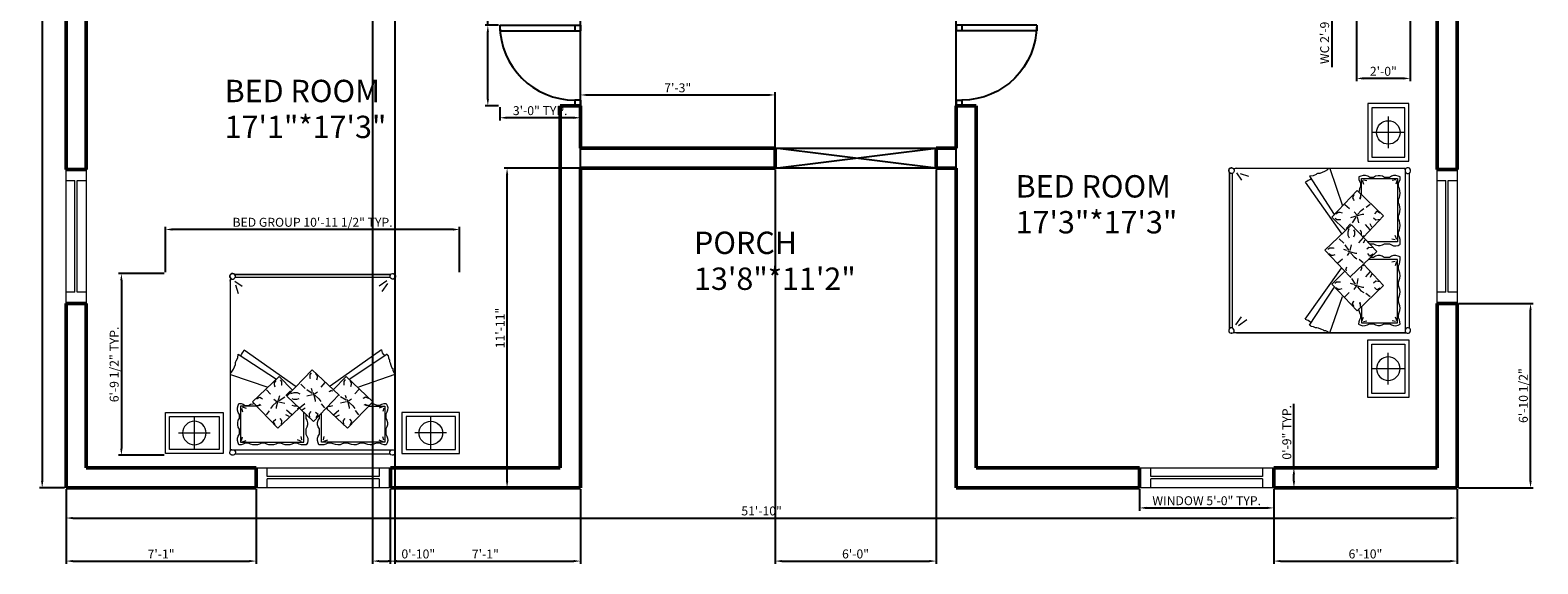
# Model space of a CAD drawing. Units: inches. Extents: x 2201 to 2875, y 1361 to 2074.
# Tile 1 of 4: x 2201 to 2875, y 1361 to 1600. Entities that reach past the tile are written whole.
import ezdxf

# ---------------------------------------------------------------- set-up
doc = ezdxf.new("R2010")
doc.units = ezdxf.units.IN
for name, color, linetype, lineweight in [('A-ANNO-DIMS', 2, 'Continuous', 18), ('A-AREA-IDEN', 7, 'Continuous', 25), ('doors', 5, 'Continuous', 25), ('furniture', 8, 'Continuous', 18), ('sliding door', 2, 'Continuous', 25), ('walls', 6, 'Continuous', 50), ('windows', 4, 'Continuous', 18)]:
    doc.layers.add(name, color=color, linetype=linetype, lineweight=lineweight)
doc.styles.get("Standard").update_dxf_attribs({"font": 'arial.ttf'})
doc.dimstyles.new('ISO-25', dxfattribs={"dimtxt": 4, "dimasz": 3, "dimexe": 1.25, "dimexo": 0.625, "dimtad": 1, "dimlunit": 3, "dimtxsty": 'Standard', "dimcen": 2.5, "dimadec": 0, "dimazin": 0, "dimtfac": 1, "dimtmove": 0, "dimatfit": 3, "dimfxl": 1, "dimarcsym": 0})

# ---------------------------------------------------------------- blocks, each defined once
blk = doc.blocks.new('d-bed-3')
at = {"color": 0, "linetype": 'ByBlock'}
for p, q in [((0, 0), (0, -0.5)), ((0.7, 0), (0, 0)), ((0.7, -0.5), (0.7, 0)), ((0.782, -0.005), (0.786, 0.008)), ((0.782, -0.005), (0.786, 0.008)), ((0.786, 0.008), (0.797, 0.017)), ((0.786, 0.008), (0.797, 0.017)), ((0.797, 0.017), (0.808, 0.021)), ((0.797, 0.017), (0.808, 0.021)), ((0.808, 0.021), (0.821, 0.021)), ((0.808, 0.021), (0.821, 0.021)), ((0.821, 0.021), (0.835, 0.014)), ((0.821, 0.021), (0.835, 0.014)), ((0.835, 0.014), (0.841, 0.008)), ((0.835, 0.014), (0.843, 0.006)), ((0.839, 0.008), (2.73, 0.008)), ((0.841, 0.008), (2.73, 0.008)), ((0.843, 0.006), (0.848, -0.008)), ((2.723, -0.008), (2.728, 0.006)), ((2.728, 0.006), (2.736, 0.014)), ((2.73, 0.008), (2.736, 0.014)), ((2.736, 0.014), (2.751, 0.021)), ((2.736, 0.014), (2.751, 0.021)), ((2.751, 0.021), (2.764, 0.021)), ((2.751, 0.021), (2.764, 0.021)), ((2.764, 0.021), (2.775, 0.017)), ((2.764, 0.021), (2.775, 0.017)), ((2.775, 0.017), (2.786, 0.008)), ((2.775, 0.017), (2.786, 0.008)), ((2.786, 0.008), (2.79, -0.005)), ((2.786, 0.008), (2.79, -0.005)), ((2.871, -0.5), (2.871, 0)), ((2.871, 0), (3.571, 0)), ((3.571, 0), (3.571, -0.5)), ((0.05, -0.05), (0.05, -0.45)), ((0.65, -0.05), (0.05, -0.05)), ((0.35, -0.058), (0.35, -0.442)), ((0.65, -0.45), (0.65, -0.05)), ((0.782, -0.019), (0.782, -0.005)), ((0.782, -0.019), (0.782, -0.005)), ((0.786, -0.03), (0.782, -0.019)), ((0.786, -0.03), (0.782, -0.019)), ((0.786, -2.094), (0.786, -0.03)), ((0.795, -0.041), (0.786, -0.03)), ((0.786, -0.032), (0.786, -2.094)), ((0.806, -0.045), (0.795, -0.041)), ((0.819, -0.045), (0.806, -0.045)), ((0.832, -0.041), (0.819, -0.045)), ((2.753, -0.045), (0.819, -0.045)), ((0.841, -0.032), (0.832, -0.041)), ((0.848, -0.021), (0.841, -0.032)), ((0.848, -0.008), (0.848, -0.021)), ((0.872, -0.159), (0.878, -0.132)), ((0.874, -0.187), (0.872, -0.159)), ((0.878, -0.132), (0.891, -0.106)), ((0.891, -0.106), (0.918, -0.108)), ((0.907, -0.575), (0.907, -0.139)), ((0.907, -0.139), (1.676, -0.139)), ((0.918, -0.108), (0.944, -0.115)), ((0.922, -0.161), (0.933, -0.204)), ((0.929, -0.143), (0.977, -0.161)), ((0.944, -0.115), (0.968, -0.128)), ((0.968, -0.128), (1.006, -0.128)), ((1.006, -0.128), (1.032, -0.117)), ((1.032, -0.117), (1.059, -0.108)), ((1.059, -0.108), (1.085, -0.106)), ((1.085, -0.106), (1.113, -0.11)), ((1.113, -0.11), (1.14, -0.117)), ((1.14, -0.117), (1.166, -0.128)), ((1.166, -0.128), (1.203, -0.128)), ((1.203, -0.128), (1.229, -0.117)), ((1.229, -0.117), (1.257, -0.108)), ((1.257, -0.108), (1.283, -0.106)), ((1.283, -0.106), (1.311, -0.11)), ((1.311, -0.11), (1.338, -0.117)), ((1.338, -0.117), (1.362, -0.128)), ((1.362, -0.128), (1.401, -0.128)), ((1.401, -0.128), (1.425, -0.117)), ((1.425, -0.117), (1.451, -0.108)), ((1.451, -0.108), (1.48, -0.106)), ((1.48, -0.106), (1.509, -0.11)), ((1.509, -0.11), (1.536, -0.117)), ((1.536, -0.117), (1.56, -0.128)), ((1.56, -0.128), (1.599, -0.128)), ((1.599, -0.128), (1.623, -0.115)), ((1.647, -0.15), (1.599, -0.166)), ((1.623, -0.115), (1.647, -0.108)), ((1.654, -0.166), (1.643, -0.209)), ((1.647, -0.108), (1.676, -0.106)), ((1.676, -0.106), (1.708, -0.106)), ((1.676, -0.139), (1.676, -0.494)), ((1.708, -0.106), (1.719, -0.132)), ((1.719, -0.132), (1.726, -0.159)), ((1.726, -0.159), (1.726, -0.187)), ((1.843, -0.159), (1.849, -0.13)), ((1.845, -0.187), (1.843, -0.159)), ((1.849, -0.13), (1.863, -0.106)), ((1.863, -0.106), (1.895, -0.106)), ((2.662, -0.137), (1.893, -0.137)), ((1.893, -0.137), (1.893, -0.505)), ((1.895, -0.106), (1.922, -0.106)), ((1.915, -0.166), (1.926, -0.209)), ((1.922, -0.106), (1.948, -0.115)), ((1.922, -0.148), (1.97, -0.166)), ((1.948, -0.115), (1.972, -0.128)), ((1.972, -0.128), (2.01, -0.128)), ((2.01, -0.128), (2.036, -0.115)), ((2.036, -0.115), (2.063, -0.108)), ((2.063, -0.108), (2.091, -0.106)), ((2.091, -0.106), (2.117, -0.108)), ((2.117, -0.108), (2.144, -0.115)), ((2.144, -0.115), (2.17, -0.128)), ((2.17, -0.128), (2.207, -0.128)), ((2.207, -0.128), (2.233, -0.115)), ((2.233, -0.115), (2.261, -0.108)), ((2.261, -0.108), (2.287, -0.106)), ((2.287, -0.106), (2.315, -0.108)), ((2.315, -0.108), (2.342, -0.115)), ((2.342, -0.115), (2.366, -0.128)), ((2.366, -0.128), (2.405, -0.128)), ((2.405, -0.128), (2.429, -0.115)), ((2.429, -0.115), (2.455, -0.108)), ((2.455, -0.108), (2.484, -0.106)), ((2.484, -0.106), (2.513, -0.108)), ((2.513, -0.108), (2.54, -0.115)), ((2.54, -0.115), (2.564, -0.128)), ((2.564, -0.128), (2.603, -0.128)), ((2.64, -0.143), (2.592, -0.159)), ((2.603, -0.128), (2.627, -0.115)), ((2.627, -0.115), (2.651, -0.106)), ((2.647, -0.159), (2.636, -0.202)), ((2.651, -0.106), (2.68, -0.106)), ((2.662, -0.575), (2.662, -0.137)), ((2.68, -0.106), (2.691, -0.13)), ((2.691, -0.13), (2.697, -0.159)), ((2.697, -0.159), (2.697, -0.187)), ((2.723, -0.021), (2.723, -0.008)), ((2.73, -0.032), (2.723, -0.021)), ((2.739, -0.041), (2.73, -0.032)), ((2.753, -0.045), (2.739, -0.041)), ((2.766, -0.045), (2.753, -0.045)), ((2.777, -0.041), (2.766, -0.045)), ((2.777, -0.041), (2.766, -0.045)), ((2.766, -0.045), (2.786, -0.045)), ((2.786, -0.045), (2.766, -0.045)), ((2.786, -0.03), (2.777, -0.041)), ((2.786, -0.03), (2.777, -0.041)), ((2.79, -0.019), (2.786, -0.03)), ((2.79, -0.019), (2.786, -0.03)), ((2.786, -2.094), (2.786, -0.045)), ((2.79, -0.005), (2.79, -0.019)), ((2.79, -0.005), (2.79, -0.019)), ((2.921, -0.45), (2.921, -0.05)), ((2.921, -0.05), (3.521, -0.05)), ((3.221, -0.058), (3.221, -0.442)), ((3.521, -0.05), (3.521, -0.45)), ((0.158, -0.25), (0.542, -0.25)), ((0.883, -0.213), (0.874, -0.187)), ((0.876, -0.349), (0.883, -0.324)), ((0.876, -0.378), (0.876, -0.349)), ((0.896, -0.237), (0.883, -0.213)), ((0.883, -0.324), (0.896, -0.299)), ((0.896, -0.299), (0.896, -0.237)), ((1.054, -0.629), (1.362, -0.308)), ((1.329, -0.351), (1.307, -0.391)), ((1.362, -0.308), (1.619, -0.553)), ((1.405, -0.347), (1.412, -0.402)), ((1.717, -0.213), (1.702, -0.237)), ((1.702, -0.237), (1.702, -0.299)), ((1.702, -0.299), (1.717, -0.324)), ((1.726, -0.187), (1.717, -0.213)), ((1.717, -0.324), (1.724, -0.349)), ((1.724, -0.349), (1.724, -0.378)), ((1.854, -0.213), (1.845, -0.187)), ((1.847, -0.349), (1.854, -0.321)), ((1.847, -0.375), (1.847, -0.349)), ((1.867, -0.237), (1.854, -0.213)), ((1.854, -0.321), (1.867, -0.297)), ((1.867, -0.297), (1.867, -0.237)), ((2.207, -0.308), (1.948, -0.553)), ((2.163, -0.344), (2.157, -0.4)), ((2.515, -0.629), (2.207, -0.308)), ((2.241, -0.351), (2.263, -0.389)), ((2.688, -0.213), (2.673, -0.237)), ((2.673, -0.237), (2.673, -0.297)), ((2.673, -0.297), (2.688, -0.321)), ((2.697, -0.187), (2.688, -0.213)), ((2.688, -0.321), (2.695, -0.349)), ((2.695, -0.349), (2.695, -0.375)), ((3.414, -0.25), (3.029, -0.25)), ((0, -0.5), (0.7, -0.5)), ((0.05, -0.45), (0.65, -0.45)), ((0.872, -0.558), (0.874, -0.529)), ((0.874, -0.529), (0.883, -0.502)), ((0.883, -0.404), (0.876, -0.378)), ((0.896, -0.428), (0.883, -0.404)), ((0.883, -0.502), (0.896, -0.478)), ((0.896, -0.478), (0.896, -0.428)), ((0.922, -0.553), (0.933, -0.511)), ((1.225, -0.472), (1.263, -0.522)), ((1.296, -0.582), (1.274, -0.549)), ((1.307, -0.391), (1.335, -0.417)), ((1.34, -0.564), (1.34, -0.549)), ((1.412, -0.402), (1.39, -0.428)), ((1.501, -0.451), (1.46, -0.472)), ((1.467, -0.713), (1.775, -0.391)), ((1.533, -0.472), (1.467, -0.527)), ((1.599, -0.549), (1.614, -0.555)), ((1.717, -0.404), (1.702, -0.428)), ((1.702, -0.428), (1.702, -0.465)), ((1.724, -0.378), (1.717, -0.404)), ((1.742, -0.435), (1.719, -0.474)), ((1.719, -0.474), (1.749, -0.5)), ((1.775, -0.391), (2.098, -0.698)), ((1.823, -0.485), (1.801, -0.511)), ((1.819, -0.431), (1.823, -0.485)), ((1.854, -0.404), (1.847, -0.375)), ((1.867, -0.428), (1.854, -0.404)), ((1.867, -0.478), (1.867, -0.428)), ((1.911, -0.533), (1.874, -0.555)), ((1.97, -0.547), (1.95, -0.555)), ((2.036, -0.472), (2.102, -0.527)), ((2.069, -0.451), (2.109, -0.472)), ((2.157, -0.4), (2.179, -0.428)), ((2.229, -0.564), (2.229, -0.547)), ((2.263, -0.389), (2.233, -0.417)), ((2.274, -0.58), (2.296, -0.547)), ((2.344, -0.472), (2.307, -0.52)), ((2.647, -0.553), (2.636, -0.509)), ((2.688, -0.404), (2.673, -0.428)), ((2.673, -0.428), (2.673, -0.476)), ((2.673, -0.476), (2.688, -0.5)), ((2.695, -0.375), (2.688, -0.404)), ((2.688, -0.5), (2.697, -0.527)), ((2.697, -0.527), (2.697, -0.555)), ((3.571, -0.5), (2.871, -0.5)), ((3.521, -0.45), (2.921, -0.45)), ((0.878, -0.584), (0.872, -0.558)), ((0.891, -0.61), (0.878, -0.584)), ((0.918, -0.607), (0.891, -0.61)), ((1.109, -0.575), (0.907, -0.575)), ((0.944, -0.601), (0.918, -0.607)), ((0.929, -0.571), (0.977, -0.553)), ((0.968, -0.589), (0.944, -0.601)), ((1.006, -0.589), (0.968, -0.589)), ((1.032, -0.6), (1.006, -0.589)), ((1.059, -0.607), (1.032, -0.6)), ((1.379, -0.936), (1.054, -0.629)), ((1.076, -0.61), (1.059, -0.607)), ((1.105, -0.586), (1.127, -0.586)), ((1.105, -0.669), (1.142, -0.685)), ((1.127, -0.586), (1.148, -0.597)), ((1.148, -0.597), (1.131, -0.586)), ((1.131, -0.586), (1.159, -0.593)), ((1.142, -0.685), (1.164, -0.674)), ((1.164, -0.674), (1.175, -0.669)), ((1.225, -0.779), (1.274, -0.724)), ((1.346, -0.625), (1.296, -0.582)), ((1.314, -0.663), (1.351, -0.636)), ((1.357, -0.625), (1.34, -0.564)), ((1.368, -0.663), (1.357, -0.625)), ((1.373, -0.629), (1.445, -0.614)), ((1.373, -0.669), (1.384, -0.707)), ((1.379, -0.647), (1.445, -0.691)), ((1.467, -0.713), (1.46, -0.707)), ((1.79, -1.019), (1.467, -0.713)), ((1.566, -0.575), (1.538, -0.586)), ((1.597, -0.575), (1.566, -0.575)), ((1.638, -0.555), (1.676, -0.605)), ((1.708, -0.665), (1.687, -0.632)), ((1.76, -0.709), (1.708, -0.665)), ((1.726, -0.745), (1.764, -0.72)), ((1.753, -0.649), (1.753, -0.632)), ((1.771, -0.709), (1.753, -0.649)), ((1.782, -0.745), (1.771, -0.709)), ((1.786, -0.713), (1.856, -0.698)), ((2.098, -0.698), (1.79, -1.019)), ((1.79, -0.731), (1.856, -0.774)), ((1.944, -0.555), (1.878, -0.61)), ((1.972, -0.741), (1.939, -0.724)), ((1.976, -0.66), (1.95, -0.671)), ((1.968, -0.575), (2.004, -0.575)), ((2.017, -0.66), (1.976, -0.66)), ((2.004, -0.575), (2.032, -0.586)), ((2.05, -0.731), (2.01, -0.741)), ((2.039, -0.671), (2.017, -0.66)), ((2.039, -0.643), (2.043, -0.64)), ((2.054, -0.761), (2.109, -0.707)), ((2.196, -0.629), (2.124, -0.612)), ((2.19, -0.645), (2.124, -0.689)), ((2.196, -0.667), (2.185, -0.707)), ((2.19, -0.936), (2.515, -0.629)), ((2.201, -0.663), (2.212, -0.623)), ((2.212, -0.623), (2.229, -0.564)), ((2.256, -0.663), (2.218, -0.634)), ((2.222, -0.623), (2.274, -0.58)), ((2.344, -0.776), (2.296, -0.722)), ((2.405, -0.674), (2.394, -0.667)), ((2.427, -0.685), (2.405, -0.674)), ((2.438, -0.586), (2.409, -0.591)), ((2.442, -0.586), (2.42, -0.597)), ((2.42, -0.597), (2.438, -0.586)), ((2.464, -0.667), (2.427, -0.685)), ((2.464, -0.586), (2.442, -0.586)), ((2.46, -0.575), (2.662, -0.575)), ((2.513, -0.605), (2.496, -0.607)), ((2.54, -0.6), (2.513, -0.605)), ((2.564, -0.586), (2.54, -0.6)), ((2.603, -0.586), (2.564, -0.586)), ((2.64, -0.569), (2.592, -0.553)), ((2.627, -0.6), (2.603, -0.586)), ((2.651, -0.607), (2.627, -0.6)), ((2.68, -0.607), (2.651, -0.607)), ((2.691, -0.584), (2.68, -0.607)), ((2.697, -0.555), (2.691, -0.584)), ((0.786, -0.961), (1.229, -0.807)), ((0.878, -1.206), (1.335, -0.906)), ((0.95, -1.261), (1.571, -0.818)), ((1.318, -0.838), (1.324, -0.812)), ((1.318, -0.86), (1.318, -0.838)), ((1.335, -0.888), (1.318, -0.86)), ((1.379, -0.936), (1.536, -0.776)), ((1.39, -0.899), (1.405, -0.877)), ((1.405, -0.834), (1.401, -0.834)), ((1.405, -0.877), (1.405, -0.834)), ((1.555, -0.767), (1.54, -0.763)), ((1.555, -0.767), (1.577, -0.756)), ((1.577, -0.756), (1.588, -0.752)), ((1.638, -0.862), (1.687, -0.807)), ((1.73, -0.921), (1.738, -0.894)), ((1.786, -0.752), (1.797, -0.79)), ((1.928, -0.845), (1.874, -0.79)), ((2.01, -0.741), (1.972, -0.741)), ((2.618, -1.261), (1.985, -0.816)), ((2.19, -0.936), (2.028, -0.77)), ((2.163, -0.876), (2.163, -0.832)), ((2.163, -0.832), (2.168, -0.832)), ((2.179, -0.897), (2.163, -0.876)), ((2.691, -1.206), (2.225, -0.906)), ((2.233, -0.886), (2.252, -0.86)), ((2.252, -0.838), (2.245, -0.809)), ((2.252, -0.86), (2.252, -0.838)), ((2.783, -0.961), (2.328, -0.807)), ((0.813, -1.012), (0.786, -0.961)), ((0.813, -1.033), (0.813, -1.012)), ((0.824, -1.041), (0.813, -1.033)), ((0.83, -1.063), (0.824, -1.041)), ((0.835, -1.075), (0.83, -1.063)), ((0.845, -1.103), (0.835, -1.075)), ((1.73, -0.943), (1.73, -0.921)), ((1.749, -0.972), (1.73, -0.943)), ((1.801, -0.983), (1.819, -0.961)), ((1.819, -0.917), (1.812, -0.917)), ((1.819, -0.961), (1.819, -0.917)), ((2.746, -1.026), (2.723, -1.081)), ((2.723, -1.081), (2.723, -1.108)), ((2.768, -0.989), (2.746, -1.026)), ((2.779, -0.983), (2.768, -0.989)), ((2.783, -0.961), (2.779, -0.983)), ((0.852, -1.119), (0.845, -1.103)), ((0.852, -1.136), (0.852, -1.119)), ((0.863, -1.162), (0.852, -1.136)), ((0.867, -1.19), (0.863, -1.162)), ((0.874, -1.195), (0.867, -1.19)), ((0.878, -1.206), (0.874, -1.195)), ((0.922, -1.202), (0.911, -1.184)), ((0.929, -1.206), (0.922, -1.202)), ((0.94, -1.224), (0.929, -1.206)), ((0.944, -1.239), (0.94, -1.224)), ((0.95, -1.261), (0.944, -1.239)), ((2.625, -1.239), (2.618, -1.261)), ((2.636, -1.224), (2.625, -1.239)), ((2.647, -1.202), (2.636, -1.224)), ((2.658, -1.184), (2.647, -1.202)), ((2.695, -1.162), (2.691, -1.206)), ((2.712, -1.125), (2.695, -1.162)), ((2.717, -1.119), (2.712, -1.125)), ((2.723, -1.108), (2.717, -1.119)), ((0.874, -2.067), (0.946, -1.969)), ((2.723, -2.05), (2.691, -1.947)), ((0.78, -2.148), (0.786, -2.135)), ((0.78, -2.148), (0.786, -2.135)), ((0.78, -2.159), (0.78, -2.148)), ((0.78, -2.148), (0.78, -2.159)), ((0.784, -2.172), (0.78, -2.159)), ((0.784, -2.172), (0.78, -2.159)), ((0.793, -2.181), (0.784, -2.172)), ((0.793, -2.181), (0.784, -2.172)), ((0.789, -2.132), (0.786, -2.094)), ((0.786, -2.094), (0.789, -2.13)), ((0.786, -2.135), (0.795, -2.126)), ((0.786, -2.135), (0.789, -2.132)), ((0.806, -2.188), (0.793, -2.181)), ((0.806, -2.188), (0.793, -2.181)), ((0.795, -2.126), (0.808, -2.121)), ((0.817, -2.188), (0.806, -2.188)), ((0.817, -2.188), (0.806, -2.188)), ((0.808, -2.121), (0.819, -2.121)), ((0.83, -2.183), (0.817, -2.188)), ((0.83, -2.183), (0.817, -2.188)), ((0.819, -2.121), (0.832, -2.128)), ((0.839, -2.174), (0.83, -2.183)), ((0.837, -2.177), (0.83, -2.183)), ((0.832, -2.128), (0.841, -2.137)), ((2.733, -2.177), (0.837, -2.177)), ((0.845, -2.161), (0.839, -2.174)), ((0.839, -2.177), (2.73, -2.177)), ((0.841, -2.137), (0.845, -2.15)), ((2.726, -2.144), (0.845, -2.144)), ((0.845, -2.15), (0.845, -2.161)), ((0.885, -2.1), (0.979, -2.034)), ((2.73, -2.094), (2.642, -2.034)), ((2.728, -2.137), (2.723, -2.15)), ((2.723, -2.15), (2.723, -2.161)), ((2.723, -2.161), (2.73, -2.174)), ((2.736, -2.128), (2.728, -2.137)), ((2.73, -2.174), (2.739, -2.183)), ((2.739, -2.183), (2.733, -2.177)), ((2.751, -2.121), (2.736, -2.128)), ((2.753, -2.188), (2.739, -2.183)), ((2.739, -2.183), (2.753, -2.188)), ((2.762, -2.121), (2.751, -2.121)), ((2.764, -2.188), (2.753, -2.188)), ((2.753, -2.188), (2.764, -2.188)), ((2.775, -2.126), (2.762, -2.121)), ((2.777, -2.181), (2.764, -2.188)), ((2.764, -2.188), (2.777, -2.181)), ((2.783, -2.135), (2.775, -2.126)), ((2.786, -2.172), (2.777, -2.181)), ((2.777, -2.181), (2.786, -2.172)), ((2.786, -2.094), (2.778, -2.13)), ((2.778, -2.13), (2.783, -2.135)), ((2.779, -2.128), (2.786, -2.094)), ((2.783, -2.135), (2.79, -2.148)), ((2.79, -2.148), (2.783, -2.135)), ((2.79, -2.159), (2.786, -2.172)), ((2.786, -2.172), (2.79, -2.159)), ((2.79, -2.148), (2.79, -2.159)), ((2.79, -2.159), (2.79, -2.148))]:
    blk.add_line(p, q, dxfattribs=at)
blk.add_ellipse((0.35, -0.25), major_axis=(-0.101, 0.101), ratio=1, dxfattribs=at)
at = {"color": 0, "linetype": 'ByBlock', "extrusion": (0, 0, -1)}
blk.add_ellipse((3.221, -0.25), major_axis=(0.101, 0.101), ratio=1, dxfattribs=at)
blk = doc.blocks.new('*D10')
at = {"layer": 'A-ANNO-DIMS', "color": 0, "lineweight": -2, "transparency": 16777216}
for p, q in [((2217.4, 1394.26), (2217.4, 1380.09)), ((2839.4, 1394.26), (2839.4, 1380.09)), ((2220.4, 1381.34), (2836.4, 1381.34))]:
    blk.add_line(p, q, dxfattribs=at)
at = {"layer": 'A-ANNO-DIMS', "color": 0, "transparency": 16777216}
for points in [[(2220.4, 1381.84), (2220.4, 1380.84), (2217.4, 1381.34)], [(2836.4, 1381.84), (2836.4, 1380.84), (2839.4, 1381.34)]]:
    blk.add_solid(points, dxfattribs=at)
at = {"layer": 'Defpoints', "color": 0, "transparency": 16777216}
for p in [(2217.4, 1394.88), (2839.4, 1394.88), (2839.4, 1381.34)]:
    blk.add_point(p, dxfattribs=at)
at = {"layer": 'A-ANNO-DIMS', "color": 0, "transparency": 16777216, "insert": (2528.4, 1384.01), "char_height": 4, "attachment_point": 5}
blk.add_mtext('51\'-10"', dxfattribs=at)
blk = doc.blocks.new('*D11')
at = {"layer": 'A-ANNO-DIMS', "color": 0, "lineweight": -2, "transparency": 16777216}
for p, q in [((2216.78, 2035.88), (2205.5, 2035.88)), ((2206.75, 2032.88), (2206.75, 1397.88)), ((2216.78, 1394.88), (2205.5, 1394.88))]:
    blk.add_line(p, q, dxfattribs=at)
at = {"layer": 'A-ANNO-DIMS', "color": 0, "transparency": 16777216}
for points in [[(2206.25, 2032.88), (2207.25, 2032.88), (2206.75, 2035.88)], [(2206.25, 1397.88), (2207.25, 1397.88), (2206.75, 1394.88)]]:
    blk.add_solid(points, dxfattribs=at)
at = {"layer": 'Defpoints', "color": 0, "transparency": 16777216}
for p in [(2217.4, 2035.88), (2206.75, 1394.88), (2217.4, 1394.88)]:
    blk.add_point(p, dxfattribs=at)
at = {"layer": 'A-ANNO-DIMS', "color": 0, "transparency": 16777216, "insert": (2204.09, 1715.38), "char_height": 4, "attachment_point": 5, "rotation": 90}
blk.add_mtext('53\'-5"', dxfattribs=at)
blk = doc.blocks.new('DOOR-SWING-36IN')
for p, q in [((33.5, 36), (33.5, 0)), ((36, 36), (33.5, 36)), ((36, 36), (36, 0)), ((2.5, 2.5), (0, 2.5)), ((0, 0), (0, 2.5)), ((2.5, 0), (2.5, 2.5)), ((36, 2.5), (33.5, 2.5)), ((2.5, 0), (0, 0)), ((36, 0), (33.5, 0))]:
    blk.add_line(p, q)
blk.add_arc((36, 2.5), 33.5, 90, 180)
blk = doc.blocks.new('WIN-60IN')
for p, q in [((0, 9), (60, 9)), ((0, 0), (0, 9)), ((5, 5), (5, 9)), ((55, 9), (55, 5)), ((60, 9), (60, 0)), ((55, 5), (5, 5)), ((5, 0), (5, 4)), ((55, 4), (5, 4)), ((55, 4), (55, 0)), ((60, 0), (0, 0))]:
    blk.add_line(p, q)
blk = doc.blocks.new('*D16')
at = {"layer": 'A-ANNO-DIMS', "color": 0, "lineweight": -2, "transparency": 16777216}
for p, q in [((2697.4, 1394.26), (2697.4, 1384.63)), ((2757.4, 1394.26), (2757.4, 1384.63)), ((2700.4, 1385.88), (2754.4, 1385.88))]:
    blk.add_line(p, q, dxfattribs=at)
at = {"layer": 'A-ANNO-DIMS', "color": 0, "transparency": 16777216}
for points in [[(2700.4, 1386.38), (2700.4, 1385.38), (2697.4, 1385.88)], [(2754.4, 1386.38), (2754.4, 1385.38), (2757.4, 1385.88)]]:
    blk.add_solid(points, dxfattribs=at)
at = {"layer": 'Defpoints', "color": 0, "transparency": 16777216}
for p in [(2697.4, 1394.88), (2757.4, 1394.88), (2757.4, 1385.88)]:
    blk.add_point(p, dxfattribs=at)
at = {"layer": 'A-ANNO-DIMS', "color": 0, "transparency": 16777216, "insert": (2727.4, 1388.58), "char_height": 4, "attachment_point": 5}
blk.add_mtext('WINDOW 5\'-0" TYP.', dxfattribs=at)
blk = doc.blocks.new('*D17')
at = {"layer": 'A-ANNO-DIMS', "color": 0, "lineweight": -2, "transparency": 16777216}
for p, q in [((2766.4, 1403.88), (2766.4, 1432.51)), ((2758.03, 1403.88), (2767.65, 1403.88)), ((2766.4, 1397.88), (2766.4, 1400.88)), ((2758.03, 1394.88), (2767.65, 1394.88))]:
    blk.add_line(p, q, dxfattribs=at)
at = {"layer": 'A-ANNO-DIMS', "color": 0, "transparency": 16777216}
for points in [[(2765.9, 1400.88), (2766.9, 1400.88), (2766.4, 1403.88)], [(2765.9, 1397.88), (2766.9, 1397.88), (2766.4, 1394.88)]]:
    blk.add_solid(points, dxfattribs=at)
at = {"layer": 'Defpoints', "color": 0, "transparency": 16777216}
for p in [(2757.4, 1403.88), (2766.4, 1403.88), (2757.4, 1394.88)]:
    blk.add_point(p, dxfattribs=at)
at = {"layer": 'A-ANNO-DIMS', "color": 0, "transparency": 16777216, "insert": (2763.74, 1419.7), "char_height": 4, "attachment_point": 5, "rotation": 90}
blk.add_mtext('0\'-9" TYP.', dxfattribs=at)
blk = doc.blocks.new('*D18')
at = {"layer": 'A-ANNO-DIMS', "color": 0, "lineweight": -2, "transparency": 16777216}
for p, q in [((2406, 1601.88), (2406, 1648.63)), ((2410.78, 1601.88), (2404.75, 1601.88)), ((2406, 1568.88), (2406, 1598.88)), ((2410.78, 1565.88), (2404.75, 1565.88))]:
    blk.add_line(p, q, dxfattribs=at)
at = {"layer": 'A-ANNO-DIMS', "color": 0, "transparency": 16777216}
for points in [[(2405.5, 1598.88), (2406.5, 1598.88), (2406, 1601.88)], [(2405.5, 1568.88), (2406.5, 1568.88), (2406, 1565.88)]]:
    blk.add_solid(points, dxfattribs=at)
at = {"layer": 'Defpoints', "color": 0, "transparency": 16777216}
for p in [(2406, 1601.88), (2411.4, 1601.88), (2411.4, 1565.88)]:
    blk.add_point(p, dxfattribs=at)
at = {"layer": 'A-ANNO-DIMS', "color": 0, "transparency": 16777216, "insert": (2403.31, 1626.76), "char_height": 4, "attachment_point": 5, "rotation": 90}
blk.add_mtext('DOOR 3\'-0" TYP.', dxfattribs=at)
blk = doc.blocks.new('*D19')
at = {"layer": 'A-ANNO-DIMS', "color": 0, "lineweight": -2, "transparency": 16777216}
for p, q in [((2411.4, 1565.26), (2411.4, 1559.23)), ((2447.4, 1565.26), (2447.4, 1559.23)), ((2444.4, 1560.48), (2414.4, 1560.48))]:
    blk.add_line(p, q, dxfattribs=at)
at = {"layer": 'A-ANNO-DIMS', "color": 0, "transparency": 16777216}
for points in [[(2414.4, 1560.98), (2414.4, 1559.98), (2411.4, 1560.48)], [(2444.4, 1560.98), (2444.4, 1559.98), (2447.4, 1560.48)]]:
    blk.add_solid(points, dxfattribs=at)
at = {"layer": 'Defpoints', "color": 0, "transparency": 16777216}
for p in [(2411.4, 1565.88), (2447.4, 1565.88), (2411.4, 1560.48)]:
    blk.add_point(p, dxfattribs=at)
at = {"layer": 'A-ANNO-DIMS', "color": 0, "transparency": 16777216, "insert": (2429.4, 1563.15), "char_height": 4, "attachment_point": 5}
blk.add_mtext('3\'-0" TYP.', dxfattribs=at)
blk = doc.blocks.new('*D20')
at = {"layer": 'A-ANNO-DIMS', "color": 0, "lineweight": -2, "transparency": 16777216}
for p, q in [((2261.88, 1491.38), (2261.88, 1511.73)), ((2390.39, 1510.48), (2264.88, 1510.48)), ((2393.39, 1491.38), (2393.39, 1511.73))]:
    blk.add_line(p, q, dxfattribs=at)
at = {"layer": 'A-ANNO-DIMS', "color": 0, "transparency": 16777216}
for points in [[(2264.88, 1510.98), (2264.88, 1509.98), (2261.88, 1510.48)], [(2390.39, 1510.98), (2390.39, 1509.98), (2393.39, 1510.48)]]:
    blk.add_solid(points, dxfattribs=at)
at = {"layer": 'Defpoints', "color": 0, "transparency": 16777216}
for p in [(2261.88, 1510.48), (2261.88, 1490.76), (2393.39, 1490.76)]:
    blk.add_point(p, dxfattribs=at)
at = {"layer": 'A-ANNO-DIMS', "color": 0, "transparency": 16777216, "insert": (2327.63, 1513.18), "char_height": 4, "attachment_point": 5}
blk.add_mtext('BED GROUP 10\'-11 1/2" TYP.', dxfattribs=at)
blk = doc.blocks.new('*D21')
at = {"layer": 'A-ANNO-DIMS', "color": 0, "lineweight": -2, "transparency": 16777216}
for p, q in [((2261.25, 1490.76), (2240.9, 1490.76)), ((2242.15, 1487.76), (2242.15, 1412.42)), ((2261.25, 1409.42), (2240.9, 1409.42))]:
    blk.add_line(p, q, dxfattribs=at)
at = {"layer": 'A-ANNO-DIMS', "color": 0, "transparency": 16777216}
for points in [[(2241.65, 1487.76), (2242.65, 1487.76), (2242.15, 1490.76)], [(2241.65, 1412.42), (2242.65, 1412.42), (2242.15, 1409.42)]]:
    blk.add_solid(points, dxfattribs=at)
at = {"layer": 'Defpoints', "color": 0, "transparency": 16777216}
for p in [(2261.88, 1490.76), (2242.15, 1409.42), (2261.88, 1409.42)]:
    blk.add_point(p, dxfattribs=at)
at = {"layer": 'A-ANNO-DIMS', "color": 0, "transparency": 16777216, "insert": (2239.46, 1450.09), "char_height": 4, "attachment_point": 5, "rotation": 90}
blk.add_mtext('6\'-9 1/2" TYP.', dxfattribs=at)
blk = doc.blocks.new('*D26')
at = {"layer": 'A-ANNO-DIMS', "color": 0, "lineweight": -2, "transparency": 16777216}
for p, q in [((2779.03, 1655.83), (2784.62, 1655.83)), ((2783.37, 1652.83), (2783.37, 1625.78)), ((2779.03, 1622.78), (2784.62, 1622.78)), ((2783.37, 1622.78), (2783.37, 1583.13))]:
    blk.add_line(p, q, dxfattribs=at)
at = {"layer": 'A-ANNO-DIMS', "color": 0, "transparency": 16777216}
for points in [[(2782.87, 1652.83), (2783.87, 1652.83), (2783.37, 1655.83)], [(2782.87, 1625.78), (2783.87, 1625.78), (2783.37, 1622.78)]]:
    blk.add_solid(points, dxfattribs=at)
at = {"layer": 'Defpoints', "color": 0, "transparency": 16777216}
for p in [(2778.41, 1655.83), (2778.41, 1622.78), (2783.37, 1622.78)]:
    blk.add_point(p, dxfattribs=at)
at = {"layer": 'A-ANNO-DIMS', "color": 0, "transparency": 16777216, "insert": (2780.67, 1601.46), "char_height": 4, "attachment_point": 5, "rotation": 90}
blk.add_mtext('WC 2\'-9" TYP.', dxfattribs=at)
blk = doc.blocks.new('*D36')
at = {"layer": 'A-ANNO-DIMS', "color": 0, "lineweight": -2, "transparency": 16777216}
for p, q in [((2217.4, 1394.26), (2217.4, 1360.83)), ((2302.4, 1394.26), (2302.4, 1360.83)), ((2220.4, 1362.08), (2299.4, 1362.08))]:
    blk.add_line(p, q, dxfattribs=at)
at = {"layer": 'A-ANNO-DIMS', "color": 0, "transparency": 16777216}
for points in [[(2220.4, 1362.58), (2220.4, 1361.58), (2217.4, 1362.08)], [(2299.4, 1362.58), (2299.4, 1361.58), (2302.4, 1362.08)]]:
    blk.add_solid(points, dxfattribs=at)
at = {"layer": 'Defpoints', "color": 0, "transparency": 16777216}
for p in [(2217.4, 1394.88), (2302.4, 1394.88), (2302.4, 1362.08)]:
    blk.add_point(p, dxfattribs=at)
at = {"layer": 'A-ANNO-DIMS', "color": 0, "transparency": 16777216, "insert": (2259.9, 1364.72), "char_height": 4, "attachment_point": 5}
blk.add_mtext('7\'-1"', dxfattribs=at)
blk = doc.blocks.new('*D37')
at = {"layer": 'A-ANNO-DIMS', "color": 0, "lineweight": -2, "transparency": 16777216}
for p, q in [((2757.4, 1394.26), (2757.4, 1360.83)), ((2839.4, 1394.26), (2839.4, 1360.83)), ((2760.4, 1362.08), (2836.4, 1362.08))]:
    blk.add_line(p, q, dxfattribs=at)
at = {"layer": 'A-ANNO-DIMS', "color": 0, "transparency": 16777216}
for points in [[(2760.4, 1362.58), (2760.4, 1361.58), (2757.4, 1362.08)], [(2836.4, 1362.58), (2836.4, 1361.58), (2839.4, 1362.08)]]:
    blk.add_solid(points, dxfattribs=at)
at = {"layer": 'Defpoints', "color": 0, "transparency": 16777216}
for p in [(2757.4, 1394.88), (2839.4, 1394.88), (2839.4, 1362.08)]:
    blk.add_point(p, dxfattribs=at)
at = {"layer": 'A-ANNO-DIMS', "color": 0, "transparency": 16777216, "insert": (2798.4, 1364.75), "char_height": 4, "attachment_point": 5}
blk.add_mtext('6\'-10"', dxfattribs=at)
blk = doc.blocks.new('*D38')
at = {"layer": 'A-ANNO-DIMS', "color": 0, "lineweight": -2, "transparency": 16777216}
for p, q in [((2840.03, 1477.38), (2873.45, 1477.38)), ((2872.2, 1397.88), (2872.2, 1474.38)), ((2840.03, 1394.88), (2873.45, 1394.88))]:
    blk.add_line(p, q, dxfattribs=at)
at = {"layer": 'A-ANNO-DIMS', "color": 0, "transparency": 16777216}
for points in [[(2871.7, 1474.38), (2872.7, 1474.38), (2872.2, 1477.38)], [(2871.7, 1397.88), (2872.7, 1397.88), (2872.2, 1394.88)]]:
    blk.add_solid(points, dxfattribs=at)
at = {"layer": 'Defpoints', "color": 0, "transparency": 16777216}
for p in [(2839.4, 1477.38), (2872.2, 1477.38), (2839.4, 1394.88)]:
    blk.add_point(p, dxfattribs=at)
at = {"layer": 'A-ANNO-DIMS', "color": 0, "transparency": 16777216, "insert": (2869.51, 1436.13), "char_height": 4, "attachment_point": 5, "rotation": 90}
blk.add_mtext('6\'-10 1/2"', dxfattribs=at)
blk = doc.blocks.new('*D45')
at = {"layer": 'A-ANNO-DIMS', "color": 0, "lineweight": -2, "transparency": 16777216}
for p, q in [((2534.4, 1537.26), (2534.4, 1360.83)), ((2606.4, 1537.26), (2606.4, 1360.83)), ((2537.4, 1362.08), (2603.4, 1362.08))]:
    blk.add_line(p, q, dxfattribs=at)
at = {"layer": 'A-ANNO-DIMS', "color": 0, "transparency": 16777216}
for points in [[(2537.4, 1362.58), (2537.4, 1361.58), (2534.4, 1362.08)], [(2603.4, 1362.58), (2603.4, 1361.58), (2606.4, 1362.08)]]:
    blk.add_solid(points, dxfattribs=at)
at = {"layer": 'Defpoints', "color": 0, "transparency": 16777216}
for p in [(2534.4, 1537.88), (2606.4, 1537.88), (2606.4, 1362.08)]:
    blk.add_point(p, dxfattribs=at)
at = {"layer": 'A-ANNO-DIMS', "color": 0, "transparency": 16777216, "insert": (2570.4, 1364.75), "char_height": 4, "attachment_point": 5}
blk.add_mtext('6\'-0"', dxfattribs=at)
blk = doc.blocks.new('*D46')
at = {"layer": 'A-ANNO-DIMS', "color": 0, "lineweight": -2, "transparency": 16777216}
for p, q in [((2447.4, 1538.51), (2447.4, 1571.93)), ((2534.4, 1538.51), (2534.4, 1571.93)), ((2450.4, 1570.68), (2531.4, 1570.68))]:
    blk.add_line(p, q, dxfattribs=at)
at = {"layer": 'A-ANNO-DIMS', "color": 0, "transparency": 16777216}
for points in [[(2450.4, 1571.18), (2450.4, 1570.18), (2447.4, 1570.68)], [(2531.4, 1571.18), (2531.4, 1570.18), (2534.4, 1570.68)]]:
    blk.add_solid(points, dxfattribs=at)
at = {"layer": 'Defpoints', "color": 0, "transparency": 16777216}
for p in [(2534.4, 1570.68), (2447.4, 1537.88), (2534.4, 1537.88)]:
    blk.add_point(p, dxfattribs=at)
at = {"layer": 'A-ANNO-DIMS', "color": 0, "transparency": 16777216, "insert": (2490.9, 1573.35), "char_height": 4, "attachment_point": 5}
blk.add_mtext('7\'-3"', dxfattribs=at)
blk = doc.blocks.new('*D47')
at = {"layer": 'A-ANNO-DIMS', "color": 0, "lineweight": -2, "transparency": 16777216}
for p, q in [((2794.4, 1610.26), (2794.4, 1576.83)), ((2818.4, 1610.26), (2818.4, 1576.83)), ((2815.4, 1578.08), (2797.4, 1578.08))]:
    blk.add_line(p, q, dxfattribs=at)
at = {"layer": 'A-ANNO-DIMS', "color": 0, "transparency": 16777216}
for points in [[(2797.4, 1578.58), (2797.4, 1577.58), (2794.4, 1578.08)], [(2815.4, 1578.58), (2815.4, 1577.58), (2818.4, 1578.08)]]:
    blk.add_solid(points, dxfattribs=at)
at = {"layer": 'Defpoints', "color": 0, "transparency": 16777216}
for p in [(2794.4, 1610.88), (2818.4, 1610.88), (2794.4, 1578.08)]:
    blk.add_point(p, dxfattribs=at)
at = {"layer": 'A-ANNO-DIMS', "color": 0, "transparency": 16777216, "insert": (2806.4, 1580.75), "char_height": 4, "attachment_point": 5}
blk.add_mtext('2\'-0"', dxfattribs=at)
blk = doc.blocks.new('*D51')
at = {"layer": 'A-ANNO-DIMS', "color": 0, "lineweight": -2, "transparency": 16777216}
for p, q in [((2354.4, 1758.26), (2354.4, 1360.83)), ((2364.4, 1758.26), (2364.4, 1360.83)), ((2357.4, 1362.08), (2361.4, 1362.08)), ((2364.4, 1362.08), (2382.39, 1362.08))]:
    blk.add_line(p, q, dxfattribs=at)
at = {"layer": 'A-ANNO-DIMS', "color": 0, "transparency": 16777216}
for points in [[(2357.4, 1362.58), (2357.4, 1361.58), (2354.4, 1362.08)], [(2361.4, 1362.58), (2361.4, 1361.58), (2364.4, 1362.08)]]:
    blk.add_solid(points, dxfattribs=at)
at = {"layer": 'Defpoints', "color": 0, "transparency": 16777216}
for p in [(2354.4, 1758.88), (2364.4, 1758.88), (2364.4, 1362.08)]:
    blk.add_point(p, dxfattribs=at)
at = {"layer": 'A-ANNO-DIMS', "color": 0, "transparency": 16777216, "insert": (2374.9, 1364.75), "char_height": 4, "attachment_point": 5}
blk.add_mtext('0\'-10"', dxfattribs=at)
blk = doc.blocks.new('*D56')
at = {"layer": 'A-ANNO-DIMS', "color": 0, "lineweight": -2, "transparency": 16777216}
for p, q in [((2447.4, 1395.51), (2447.4, 2069.93)), ((2615.4, 1395.51), (2615.4, 2069.93)), ((2450.4, 2068.68), (2612.4, 2068.68))]:
    blk.add_line(p, q, dxfattribs=at)
at = {"layer": 'A-ANNO-DIMS', "color": 0, "transparency": 16777216}
for points in [[(2450.4, 2069.18), (2450.4, 2068.18), (2447.4, 2068.68)], [(2612.4, 2069.18), (2612.4, 2068.18), (2615.4, 2068.68)]]:
    blk.add_solid(points, dxfattribs=at)
at = {"layer": 'Defpoints', "color": 0, "transparency": 16777216}
for p in [(2615.4, 2068.68), (2447.4, 1394.88), (2615.4, 1394.88)]:
    blk.add_point(p, dxfattribs=at)
at = {"layer": 'A-ANNO-DIMS', "color": 0, "transparency": 16777216, "insert": (2531.4, 2071.35), "char_height": 4, "attachment_point": 5}
blk.add_mtext('14\'-0"', dxfattribs=at)
blk = doc.blocks.new('*D57')
at = {"layer": 'A-ANNO-DIMS', "color": 0, "lineweight": -2, "transparency": 16777216}
for p, q in [((2446.78, 1537.88), (2413.35, 1537.88)), ((2414.6, 1397.88), (2414.6, 1534.88)), ((2446.78, 1394.88), (2413.35, 1394.88))]:
    blk.add_line(p, q, dxfattribs=at)
at = {"layer": 'A-ANNO-DIMS', "color": 0, "transparency": 16777216}
for points in [[(2414.1, 1534.88), (2415.1, 1534.88), (2414.6, 1537.88)], [(2414.1, 1397.88), (2415.1, 1397.88), (2414.6, 1394.88)]]:
    blk.add_solid(points, dxfattribs=at)
at = {"layer": 'Defpoints', "color": 0, "transparency": 16777216}
for p in [(2414.6, 1537.88), (2447.4, 1537.88), (2447.4, 1394.88)]:
    blk.add_point(p, dxfattribs=at)
at = {"layer": 'A-ANNO-DIMS', "color": 0, "transparency": 16777216, "insert": (2411.97, 1466.38), "char_height": 4, "attachment_point": 5, "rotation": 90}
blk.add_mtext('11\'-11"', dxfattribs=at)
blk = doc.blocks.new('*D58')
at = {"layer": 'A-ANNO-DIMS', "color": 0, "lineweight": -2, "transparency": 16777216}
for p, q in [((2362.4, 1394.26), (2362.4, 1360.83)), ((2447.4, 1394.26), (2447.4, 1360.83)), ((2365.4, 1362.08), (2444.4, 1362.08))]:
    blk.add_line(p, q, dxfattribs=at)
at = {"layer": 'A-ANNO-DIMS', "color": 0, "transparency": 16777216}
for points in [[(2365.4, 1362.58), (2365.4, 1361.58), (2362.4, 1362.08)], [(2444.4, 1362.58), (2444.4, 1361.58), (2447.4, 1362.08)]]:
    blk.add_solid(points, dxfattribs=at)
at = {"layer": 'Defpoints', "color": 0, "transparency": 16777216}
for p in [(2362.4, 1394.88), (2447.4, 1394.88), (2447.4, 1362.08)]:
    blk.add_point(p, dxfattribs=at)
at = {"layer": 'A-ANNO-DIMS', "color": 0, "transparency": 16777216, "insert": (2404.9, 1364.72), "char_height": 4, "attachment_point": 5}
blk.add_mtext('7\'-1"', dxfattribs=at)

msp = doc.modelspace()

# ---------------------------------------------------------------- linework, layer by layer
at = {"layer": 'sliding door'}
for p, q in [((2606.403, 1537.883), (2534.403, 1546.883)), ((2534.403, 1537.883), (2606.403, 1546.883))]:
    msp.add_line(p, q, dxfattribs=at)
msp.add_lwpolyline([(2534.403, 1546.883), (2606.403, 1546.883), (2606.403, 1537.883), (2534.403, 1537.883)], close=True, dxfattribs=at)
at = {"layer": 'walls'}
for p, q in [((2217.403, 1891.383), (2217.403, 1537.383)), ((2839.403, 1653.383), (2839.403, 1537.383)), ((2226.403, 1610.883), (2226.403, 1537.383)), ((2830.403, 1610.883), (2830.403, 1537.383)), ((2438.403, 1565.883), (2438.403, 1403.883)), ((2438.403, 1565.883), (2447.403, 1565.883)), ((2447.403, 1565.883), (2447.403, 1546.883)), ((2615.403, 1565.883), (2624.403, 1565.883)), ((2615.403, 1565.883), (2615.403, 1546.883)), ((2624.403, 1565.883), (2624.403, 1403.883)), ((2447.403, 1546.883), (2534.403, 1546.883)), ((2534.403, 1546.883), (2534.403, 1537.883)), ((2606.403, 1546.883), (2606.403, 1537.883)), ((2606.403, 1546.883), (2615.403, 1546.883)), ((2226.403, 1537.383), (2217.403, 1537.383)), ((2447.403, 1537.883), (2534.403, 1537.883)), ((2447.403, 1537.883), (2447.403, 1394.883)), ((2606.403, 1537.883), (2615.403, 1537.883)), ((2615.403, 1537.883), (2615.403, 1394.883)), ((2839.403, 1537.383), (2830.403, 1537.383)), ((2217.403, 1477.383), (2217.403, 1394.883)), ((2226.403, 1477.383), (2217.403, 1477.383)), ((2226.403, 1477.383), (2226.403, 1403.883)), ((2830.403, 1477.383), (2830.403, 1403.883)), ((2839.403, 1477.383), (2830.403, 1477.383)), ((2839.403, 1477.383), (2839.403, 1394.883)), ((2226.403, 1403.883), (2302.403, 1403.883)), ((2302.403, 1394.883), (2302.403, 1403.883)), ((2362.403, 1394.883), (2362.403, 1403.883)), ((2362.403, 1403.883), (2438.403, 1403.883)), ((2624.403, 1403.883), (2697.403, 1403.883)), ((2697.403, 1394.883), (2697.403, 1403.883)), ((2757.403, 1394.883), (2757.403, 1403.883)), ((2757.403, 1403.883), (2830.403, 1403.883)), ((2217.403, 1394.883), (2302.403, 1394.883)), ((2362.403, 1394.883), (2447.403, 1394.883)), ((2615.403, 1394.883), (2697.403, 1394.883)), ((2757.403, 1394.883), (2839.403, 1394.883))]:
    msp.add_line(p, q, dxfattribs=at)

# ---------------------------------------------------------------- block references
at = {"layer": 'doors', "rotation": 89.99999999999943}
msp.add_blockref('DOOR-SWING-36IN', (2447.402, 1565.883), dxfattribs=at)
at = {"layer": 'doors', "extrusion": (0, 0, -1), "zscale": -1, "rotation": 90.00000000000063}
msp.add_blockref('DOOR-SWING-36IN', (-2615.403, 1565.883), dxfattribs=at)
at = {"layer": 'furniture', "yscale": 36.82314656981208, "zscale": 36.82314656981208}
for p, xscale, rotation in [((2817.816, 1435.294), -36.82314656981208, 270), ((2393.386, 1410.199), 36.82314656981208, 180)]:
    msp.add_blockref('d-bed-3', p, dxfattribs=dict(at, xscale=xscale, rotation=rotation))
at = {"layer": 'windows', "rotation": 270.0000000000003}
for p in [(2217.403, 1537.382), (2830.403, 1537.382)]:
    msp.add_blockref('WIN-60IN', p, dxfattribs=at)
at = {"layer": 'windows'}
for p in [(2302.403, 1394.883), (2697.403, 1394.883)]:
    msp.add_blockref('WIN-60IN', p, dxfattribs=at)

# ---------------------------------------------------------------- texts
at = {"layer": 'A-AREA-IDEN'}
for s, p in [('BED ROOM', (2288.318, 1567.454)), ('17\'1"*17\'3"', (2288.318, 1551.39)), ('BED ROOM', (2641.978, 1524.788)), ('17\'3"*17\'3" ', (2641.978, 1508.724)), ('PORCH', (2498.19, 1499.506)), ('13\'8"*11\'2"', (2498.19, 1483.442))]:
    msp.add_text(s, height=10, dxfattribs=at).set_placement(p)

# ---------------------------------------------------------------- dimensions: what is measured, and where the dimension line sits
at = {"layer": 'A-ANNO-DIMS'}
for base, p1, p2, override, picture, middle in [((2615.403, 2068.683), (2447.403, 1394.883), (2615.403, 1394.883), {"dimdec": 1, "dimlfac": 1, "dimrnd": 0, "dimzin": 1, "dimdsep": 46, "dimlunit": 4, "dimfrac": 2}, '*D56', (2531.403, 2071.35)), ((2364.403, 1362.083), (2354.403, 1758.883), (2364.403, 1758.883), {"dimdec": 1, "dimlfac": 1, "dimrnd": 0, "dimzin": 1, "dimdsep": 46, "dimlunit": 4, "dimfrac": 2}, '*D51', (2374.898, 1364.75)), ((2606.403, 1362.083), (2534.403, 1537.883), (2606.403, 1537.883), {"dimdec": 1, "dimlfac": 1, "dimrnd": 0, "dimzin": 1, "dimdsep": 46, "dimlunit": 4, "dimfrac": 2}, '*D45', (2570.403, 1364.75)), ((2839.403, 1381.344), (2217.403, 1394.883), (2839.403, 1394.883), {"dimclrd": 0, "dimclre": 0, "dimclrt": 0}, '*D10', (2528.403, 1384.011)), ((2302.403, 1362.083), (2217.403, 1394.883), (2302.403, 1394.883), {"dimdec": 1, "dimlfac": 1, "dimrnd": 0, "dimzin": 1, "dimdsep": 46, "dimlunit": 4, "dimfrac": 2}, '*D36', (2259.903, 1364.716)), ((2447.403, 1362.083), (2362.403, 1394.883), (2447.403, 1394.883), {"dimdec": 1, "dimlfac": 1, "dimrnd": 0, "dimzin": 1, "dimdsep": 46, "dimlunit": 4, "dimfrac": 2}, '*D58', (2404.903, 1364.716)), ((2839.403, 1362.083), (2757.403, 1394.883), (2839.403, 1394.883), {"dimdec": 1, "dimlfac": 1, "dimrnd": 0, "dimzin": 1, "dimdsep": 46, "dimlunit": 4, "dimfrac": 2}, '*D37', (2798.403, 1364.75))]:
    dim = msp.add_linear_dim(base=base, p1=p1, p2=p2, dimstyle='ISO-25', override=override, dxfattribs=at)
    dim.commit()
    dim.dimension.update_dxf_attribs({"geometry": picture, "text_midpoint": middle})
for base, p1, p2, angle, override, picture, middle in [((2206.755, 1394.883), (2217.403, 2035.883), (2217.403, 1394.883), 90, {"dimclrd": 0, "dimclre": 0, "dimclrt": 0}, '*D11', (2204.086, 1715.383)), ((2794.403, 1578.083), (2818.403, 1610.883), (2794.403, 1610.883), 180, {"dimdec": 1, "dimlfac": 1, "dimrnd": 0, "dimzin": 1, "dimdsep": 46, "dimlunit": 4, "dimfrac": 2}, '*D47', (2806.403, 1580.75)), ((2534.403, 1570.683), (2447.403, 1537.883), (2534.403, 1537.883), 0, {"dimdec": 1, "dimlfac": 1, "dimrnd": 0, "dimzin": 1, "dimdsep": 46, "dimlunit": 4, "dimfrac": 2}, '*D46', (2490.903, 1573.351)), ((2414.603, 1537.883), (2447.403, 1394.883), (2447.403, 1537.883), 90, {"dimdec": 1, "dimlfac": 1, "dimrnd": 0, "dimzin": 1, "dimdsep": 46, "dimlunit": 4, "dimfrac": 2}, '*D57', (2411.97, 1466.383)), ((2872.203, 1477.383), (2839.403, 1394.883), (2839.403, 1477.383), 90, {"dimdec": 1, "dimlfac": 1, "dimrnd": 0, "dimzin": 1, "dimdsep": 46, "dimlunit": 4, "dimfrac": 2}, '*D38', (2869.51, 1436.133))]:
    dim = msp.add_linear_dim(base=base, p1=p1, p2=p2, angle=angle, dimstyle='ISO-25', override=override, dxfattribs=at)
    dim.commit()
    dim.dimension.update_dxf_attribs({"geometry": picture, "text_midpoint": middle})
for base, p1, p2, angle, text, picture, middle in [((2783.367, 1622.784), (2778.41, 1655.831), (2778.41, 1622.784), 270, 'WC <> TYP.', '*D26', (2780.673, 1601.456)), ((2406.003, 1601.883), (2411.403, 1565.883), (2411.403, 1601.883), 90, 'DOOR <> TYP.', '*D18', (2403.307, 1626.757)), ((2411.403, 1560.483), (2447.403, 1565.883), (2411.403, 1565.883), 180, '<> TYP.', '*D19', (2429.403, 1563.151)), ((2261.877, 1510.484), (2393.386, 1490.758), (2261.877, 1490.758), 180, 'BED GROUP <> TYP.', '*D20', (2327.631, 1513.179)), ((2242.15, 1409.423), (2261.877, 1490.758), (2261.877, 1409.423), 270, '<> TYP.', '*D21', (2239.457, 1450.091)), ((2766.403, 1403.883), (2757.403, 1394.883), (2757.403, 1403.883), 90, '<> TYP.', '*D17', (2763.735, 1419.699))]:
    dim = msp.add_linear_dim(base=base, p1=p1, p2=p2, angle=angle, text=text, dimstyle='ISO-25', override={"dimdec": 1, "dimlfac": 1, "dimrnd": 0, "dimzin": 1, "dimdsep": 46, "dimlunit": 4, "dimfrac": 2}, dxfattribs=at)
    dim.commit()
    dim.dimension.update_dxf_attribs({"geometry": picture, "text_midpoint": middle})
dim = msp.add_linear_dim(base=(2757.403, 1385.883), p1=(2697.403, 1394.883), p2=(2757.403, 1394.883), text='WINDOW <> TYP.', dimstyle='ISO-25', override={"dimdec": 1, "dimlfac": 1, "dimrnd": 0, "dimzin": 1, "dimdsep": 46, "dimlunit": 4, "dimfrac": 2}, dxfattribs=at)
dim.commit()
dim.dimension.update_dxf_attribs({"geometry": '*D16', "text_midpoint": (2727.403, 1388.577)})

doc.saveas('drawing.dxf')
